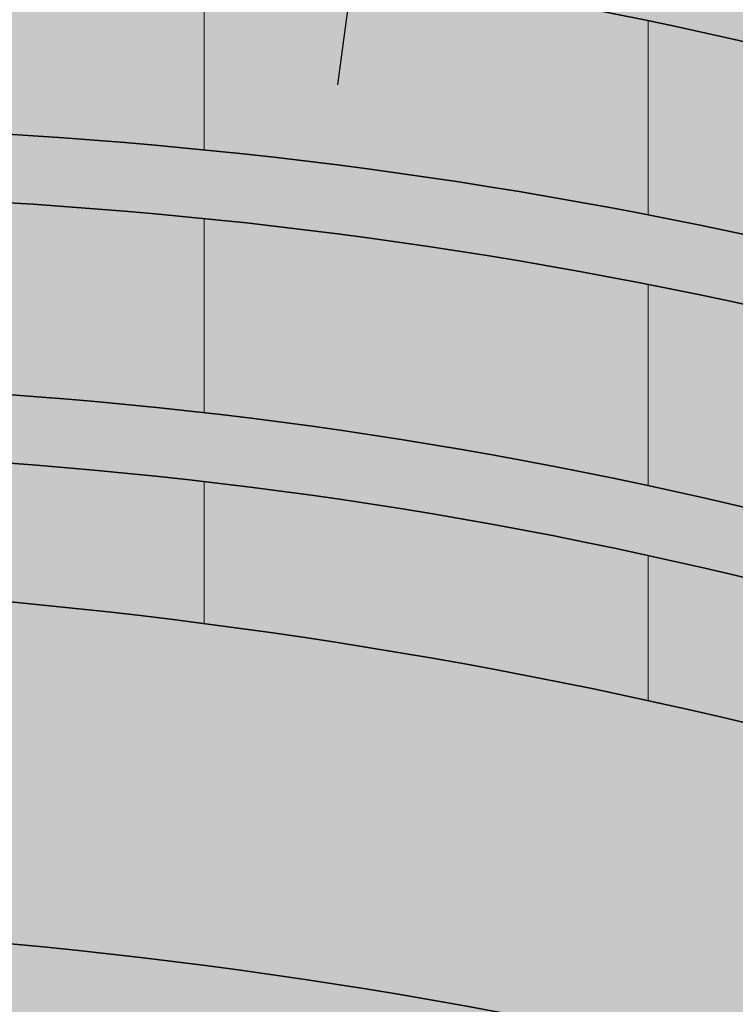
# Model space of a CAD drawing. Units: millimetres. Extents: x 130 to 1021, y 147 to 699.
# Tile 25 of 40: x 442 to 463, y 477 to 505. Entities that reach past the tile are written whole.
import ezdxf

# ---------------------------------------------------------------- set-up
doc = ezdxf.new("R2010")
doc.units = ezdxf.units.MM
doc.header["$MEASUREMENT"] = 0
for name, color, linetype, lineweight in [('A-ANNO-DIMS', 2, 'Continuous', 18), ('A-ELEV', 7, 'Continuous', 35), ('A-ELEV-PATT', 9, 'Continuous', 13), ('A-ELEV-RAIL', 6, 'Continuous', 18)]:
    doc.layers.add(name, color=color, linetype=linetype, lineweight=lineweight)
doc.styles.get("Standard").update_dxf_attribs({"font": 'arial.ttf'})
doc.dimstyles.get("Standard").update_dxf_attribs({"dimtxt": 20, "dimasz": 10, "dimexe": 10, "dimexo": 10, "dimgap": 5, "dimtad": 0, "dimtih": 1, "dimtoh": 1, "dimdec": 0, "dimzin": 0, "dimdsep": 46, "dimtxsty": 'Standard', "dimcen": 5, "dimadec": 0, "dimazin": 0, "dimtfac": 1, "dimtdec": 0, "dimtofl": 0, "dimtmove": 0, "dimatfit": 3, "dimfxl": 1, "dimtolj": 1, "dimtzin": 0, "dimarcsym": 0})

# ---------------------------------------------------------------- blocks, each defined once
blk = doc.blocks.new('*D11')
at = {"layer": 'A-ANNO-DIMS', "color": 0, "lineweight": -2, "transparency": 16777216}
for p, q in [((737.374, 648.699), (737.374, 149.739)), ((299.374, 566.947), (299.374, 149.739)), ((309.374, 159.739), (490.857, 159.739)), ((727.374, 159.739), (545.891, 159.739))]:
    blk.add_line(p, q, dxfattribs=at)
at = {"layer": 'A-ANNO-DIMS', "color": 0, "transparency": 16777216}
for points in [[(309.374, 161.406), (309.374, 158.073), (299.374, 159.739)], [(727.374, 161.406), (727.374, 158.073), (737.374, 159.739)]]:
    blk.add_solid(points, dxfattribs=at)
at = {"layer": 'Defpoints', "color": 0, "transparency": 16777216}
for p in [(737.374, 658.699), (299.374, 576.947), (737.374, 159.739)]:
    blk.add_point(p, dxfattribs=at)
at = {"layer": 'A-ANNO-DIMS', "color": 0, "transparency": 16777216, "insert": (518.374, 159.739), "char_height": 20, "attachment_point": 5}
blk.add_mtext('\\A1;438', dxfattribs=at)
blk = doc.blocks.new('*D12')
at = {"layer": 'A-ANNO-DIMS', "color": 0, "lineweight": -2, "transparency": 16777216}
for p, q in [((477.374, 661.947), (265.074, 661.947)), ((275.074, 651.947), (275.074, 438.205)), ((275.074, 194.039), (275.074, 407.782)), ((357.163, 184.039), (265.074, 184.039))]:
    blk.add_line(p, q, dxfattribs=at)
at = {"layer": 'A-ANNO-DIMS', "color": 0, "transparency": 16777216}
for points in [[(273.407, 651.947), (276.74, 651.947), (275.074, 661.947)], [(273.407, 194.039), (276.74, 194.039), (275.074, 184.039)]]:
    blk.add_solid(points, dxfattribs=at)
at = {"layer": 'Defpoints', "color": 0, "transparency": 16777216}
for p in [(275.074, 661.947), (487.374, 661.947), (367.163, 184.039)]:
    blk.add_point(p, dxfattribs=at)
at = {"layer": 'A-ANNO-DIMS', "color": 0, "transparency": 16777216, "insert": (275.074, 422.993), "char_height": 20, "attachment_point": 5}
blk.add_mtext('\\A1;477.9', dxfattribs=at)
blk = doc.blocks.new('*D16')
at = {"layer": 'A-ANNO-DIMS', "color": 0, "lineweight": -2, "transparency": 16777216}
for p, q in [((357.941, 411.947), (357.941, 696.247)), ((363.922, 579.884), (363.922, 696.247)), ((347.941, 686.247), (337.941, 686.247)), ((373.922, 686.247), (383.922, 686.247))]:
    blk.add_line(p, q, dxfattribs=at)
at = {"layer": 'A-ANNO-DIMS', "color": 0, "transparency": 16777216}
for points in [[(347.941, 687.914), (347.941, 684.581), (357.941, 686.247)], [(373.922, 687.914), (373.922, 684.581), (363.922, 686.247)]]:
    blk.add_solid(points, dxfattribs=at)
at = {"layer": 'Defpoints', "color": 0, "transparency": 16777216}
for p in [(363.922, 686.247), (363.922, 569.884), (357.941, 401.947)]:
    blk.add_point(p, dxfattribs=at)
at = {"layer": 'A-ANNO-DIMS', "color": 0, "transparency": 16777216, "insert": (420.737, 686.247), "char_height": 20, "attachment_point": 5}
blk.add_mtext('\\A1;5.981', dxfattribs=at)
blk = doc.blocks.new('*D17')
at = {"layer": 'A-ANNO-DIMS', "color": 0, "lineweight": -2, "transparency": 16777216}
for p, q in [((363.922, 579.884), (363.922, 696.247)), ((375.85, 490.216), (375.85, 696.247)), ((353.922, 686.247), (343.922, 686.247)), ((385.85, 686.247), (395.85, 686.247))]:
    blk.add_line(p, q, dxfattribs=at)
at = {"layer": 'A-ANNO-DIMS', "color": 0, "transparency": 16777216}
for points in [[(353.922, 687.914), (353.922, 684.581), (363.922, 686.247)], [(385.85, 687.914), (385.85, 684.581), (375.85, 686.247)]]:
    blk.add_solid(points, dxfattribs=at)
at = {"layer": 'Defpoints', "color": 0, "transparency": 16777216}
for p in [(375.85, 686.247), (363.922, 569.884), (375.85, 480.216)]:
    blk.add_point(p, dxfattribs=at)
at = {"layer": 'A-ANNO-DIMS', "color": 0, "transparency": 16777216, "insert": (441.444, 686.247), "char_height": 20, "attachment_point": 5}
blk.add_mtext('\\A1;11.928', dxfattribs=at)
blk = doc.blocks.new('*D18')
at = {"layer": 'A-ANNO-DIMS', "color": 0, "lineweight": -2, "transparency": 16777216}
for p, q in [((375.85, 490.216), (375.85, 696.247)), ((382.374, 388.947), (382.374, 696.247)), ((365.85, 686.247), (355.85, 686.247)), ((392.374, 686.247), (402.374, 686.247))]:
    blk.add_line(p, q, dxfattribs=at)
at = {"layer": 'A-ANNO-DIMS', "color": 0, "transparency": 16777216}
for points in [[(365.85, 687.914), (365.85, 684.581), (375.85, 686.247)], [(392.374, 687.914), (392.374, 684.581), (382.374, 686.247)]]:
    blk.add_solid(points, dxfattribs=at)
at = {"layer": 'Defpoints', "color": 0, "transparency": 16777216}
for p in [(382.374, 686.247), (375.85, 480.216), (382.374, 378.947)]:
    blk.add_point(p, dxfattribs=at)
at = {"layer": 'A-ANNO-DIMS', "color": 0, "transparency": 16777216, "insert": (441.132, 686.247), "char_height": 20, "attachment_point": 5}
blk.add_mtext('\\A1;6.524', dxfattribs=at)
blk = doc.blocks.new('*D19')
at = {"layer": 'A-ANNO-DIMS', "color": 0, "lineweight": -2, "transparency": 16777216}
for p, q in [((382.374, 388.947), (382.374, 696.247)), ((414.652, 510.881), (414.652, 696.247)), ((392.374, 686.247), (404.652, 686.247)), ((414.652, 686.247), (424.652, 686.247))]:
    blk.add_line(p, q, dxfattribs=at)
at = {"layer": 'A-ANNO-DIMS', "color": 0, "transparency": 16777216}
for points in [[(392.374, 687.914), (392.374, 684.581), (382.374, 686.247)], [(404.652, 687.914), (404.652, 684.581), (414.652, 686.247)]]:
    blk.add_solid(points, dxfattribs=at)
at = {"layer": 'Defpoints', "color": 0, "transparency": 16777216}
for p in [(414.652, 686.247), (414.652, 500.881), (382.374, 378.947)]:
    blk.add_point(p, dxfattribs=at)
at = {"layer": 'A-ANNO-DIMS', "color": 0, "transparency": 16777216, "insert": (463.411, 686.247), "char_height": 20, "attachment_point": 5}
blk.add_mtext('\\A1;32.28', dxfattribs=at)
blk = doc.blocks.new('*D20')
at = {"layer": 'A-ANNO-DIMS', "color": 0, "lineweight": -2, "transparency": 16777216}
for p, q in [((414.652, 510.881), (414.652, 696.247)), ((432.374, 388.947), (432.374, 696.247)), ((404.652, 686.247), (394.652, 686.247)), ((442.374, 686.247), (452.374, 686.247))]:
    blk.add_line(p, q, dxfattribs=at)
at = {"layer": 'A-ANNO-DIMS', "color": 0, "transparency": 16777216}
for points in [[(404.652, 687.914), (404.652, 684.581), (414.652, 686.247)], [(442.374, 687.914), (442.374, 684.581), (432.374, 686.247)]]:
    blk.add_solid(points, dxfattribs=at)
at = {"layer": 'Defpoints', "color": 0, "transparency": 16777216}
for p in [(432.374, 686.247), (414.652, 500.881), (432.374, 378.947)]:
    blk.add_point(p, dxfattribs=at)
at = {"layer": 'A-ANNO-DIMS', "color": 0, "transparency": 16777216, "insert": (490.075, 686.247), "char_height": 20, "attachment_point": 5}
blk.add_mtext('\\A1;17.72', dxfattribs=at)
blk = doc.blocks.new('*D21')
at = {"layer": 'A-ANNO-DIMS', "color": 0, "lineweight": -2, "transparency": 16777216}
for p, q in [((432.374, 388.947), (432.374, 696.247)), ((447.374, 656.947), (447.374, 696.247)), ((422.374, 686.247), (412.374, 686.247)), ((457.374, 686.247), (467.374, 686.247))]:
    blk.add_line(p, q, dxfattribs=at)
at = {"layer": 'A-ANNO-DIMS', "color": 0, "transparency": 16777216}
for points in [[(422.374, 687.914), (422.374, 684.581), (432.374, 686.247)], [(457.374, 687.914), (457.374, 684.581), (447.374, 686.247)]]:
    blk.add_solid(points, dxfattribs=at)
at = {"layer": 'Defpoints', "color": 0, "transparency": 16777216}
for p in [(447.374, 686.247), (447.374, 646.947), (432.374, 378.947)]:
    blk.add_point(p, dxfattribs=at)
at = {"layer": 'A-ANNO-DIMS', "color": 0, "transparency": 16777216, "insert": (485.832, 686.247), "char_height": 20, "attachment_point": 5}
blk.add_mtext('\\A1;15', dxfattribs=at)
blk = doc.blocks.new('*D22')
at = {"layer": 'A-ANNO-DIMS', "color": 0, "lineweight": -2, "transparency": 16777216}
for p, q in [((447.374, 656.947), (447.374, 696.247)), ((466.767, 403.947), (466.767, 696.247)), ((437.374, 686.247), (427.374, 686.247)), ((476.767, 686.247), (486.767, 686.247))]:
    blk.add_line(p, q, dxfattribs=at)
at = {"layer": 'A-ANNO-DIMS', "color": 0, "transparency": 16777216}
for points in [[(437.374, 687.914), (437.374, 684.581), (447.374, 686.247)], [(476.767, 687.914), (476.767, 684.581), (466.767, 686.247)]]:
    blk.add_solid(points, dxfattribs=at)
at = {"layer": 'Defpoints', "color": 0, "transparency": 16777216}
for p in [(466.767, 686.247), (447.374, 646.947), (466.767, 393.947)]:
    blk.add_point(p, dxfattribs=at)
at = {"layer": 'A-ANNO-DIMS', "color": 0, "transparency": 16777216, "insert": (532.34, 686.247), "char_height": 20, "attachment_point": 5}
blk.add_mtext('\\A1;19.393', dxfattribs=at)
blk = doc.blocks.new('*D23')
at = {"layer": 'A-ANNO-DIMS', "color": 0, "lineweight": -2, "transparency": 16777216}
for p, q in [((466.767, 403.947), (466.767, 696.247)), ((475.988, 209.039), (475.988, 696.247)), ((456.767, 686.247), (446.767, 686.247)), ((485.988, 686.247), (495.988, 686.247))]:
    blk.add_line(p, q, dxfattribs=at)
at = {"layer": 'A-ANNO-DIMS', "color": 0, "transparency": 16777216}
for points in [[(456.767, 687.914), (456.767, 684.581), (466.767, 686.247)], [(485.988, 687.914), (485.988, 684.581), (475.988, 686.247)]]:
    blk.add_solid(points, dxfattribs=at)
at = {"layer": 'Defpoints', "color": 0, "transparency": 16777216}
for p in [(475.988, 686.247), (466.767, 393.947), (475.988, 199.039)]:
    blk.add_point(p, dxfattribs=at)
at = {"layer": 'A-ANNO-DIMS', "color": 0, "transparency": 16777216, "insert": (534.631, 686.247), "char_height": 20, "attachment_point": 5}
blk.add_mtext('\\A1;9.222', dxfattribs=at)
blk = doc.blocks.new('*D24')
at = {"layer": 'A-ANNO-DIMS', "color": 0, "lineweight": -2, "transparency": 16777216}
for p, q in [((475.988, 209.039), (475.988, 696.247)), ((487.374, 671.947), (487.374, 696.247)), ((465.988, 686.247), (455.988, 686.247)), ((497.374, 686.247), (507.374, 686.247))]:
    blk.add_line(p, q, dxfattribs=at)
at = {"layer": 'A-ANNO-DIMS', "color": 0, "transparency": 16777216}
for points in [[(465.988, 687.914), (465.988, 684.581), (475.988, 686.247)], [(497.374, 687.914), (497.374, 684.581), (487.374, 686.247)]]:
    blk.add_solid(points, dxfattribs=at)
at = {"layer": 'Defpoints', "color": 0, "transparency": 16777216}
for p in [(487.374, 686.247), (487.374, 661.947), (475.988, 199.039)]:
    blk.add_point(p, dxfattribs=at)
at = {"layer": 'A-ANNO-DIMS', "color": 0, "transparency": 16777216, "insert": (553.022, 686.247), "char_height": 20, "attachment_point": 5}
blk.add_mtext('\\A1;11.385', dxfattribs=at)
blk = doc.blocks.new('*D65')
at = {"layer": 'A-ANNO-DIMS', "color": 0, "lineweight": -2, "transparency": 16777216}
for p, q in [((495.463, 509.127), (472.508, 423.108)), ((505.463, 509.127), (495.463, 509.127)), ((427.374, 248.979), (427.374, 258.979)), ((422.374, 253.979), (432.374, 253.979))]:
    blk.add_line(p, q, dxfattribs=at)
at = {"layer": 'A-ANNO-DIMS', "color": 0, "transparency": 16777216}
blk.add_solid([(470.898, 423.538), (474.118, 422.679), (469.93, 413.447)], dxfattribs=at)
at = {"layer": 'Defpoints', "color": 0, "transparency": 16777216}
for p in [(469.93, 413.447), (427.374, 253.979)]:
    blk.add_point(p, dxfattribs=at)
at = {"layer": 'A-ANNO-DIMS', "color": 0, "transparency": 16777216, "insert": (561.623, 509.127), "char_height": 20, "attachment_point": 5}
blk.add_mtext('\\A1;R165.05', dxfattribs=at)
blk = doc.blocks.new('*D67')
at = {"layer": 'A-ANNO-DIMS', "color": 0, "lineweight": -2, "transparency": 16777216}
for p, q in [((479.756, 492.431), (462.144, 412.223)), ((489.756, 492.431), (479.756, 492.431)), ((427.07, 247.496), (427.07, 257.496)), ((422.07, 252.496), (432.07, 252.496))]:
    blk.add_line(p, q, dxfattribs=at)
at = {"layer": 'A-ANNO-DIMS', "color": 0, "transparency": 16777216}
blk.add_solid([(460.516, 412.58), (463.772, 411.865), (459.999, 402.455)], dxfattribs=at)
at = {"layer": 'Defpoints', "color": 0, "transparency": 16777216}
for p in [(459.999, 402.455), (427.07, 252.496)]:
    blk.add_point(p, dxfattribs=at)
at = {"layer": 'A-ANNO-DIMS', "color": 0, "transparency": 16777216, "insert": (545.841, 492.431), "char_height": 20, "attachment_point": 5}
blk.add_mtext('\\A1;R153.53', dxfattribs=at)
blk = doc.blocks.new('*D69')
at = {"layer": 'A-ANNO-DIMS', "color": 0, "lineweight": -2, "transparency": 16777216}
for p, q in [((507.746, 572.261), (483.091, 501.813)), ((517.746, 572.261), (507.746, 572.261)), ((433.191, 354.23), (433.191, 364.23)), ((428.191, 359.23), (438.191, 359.23))]:
    blk.add_line(p, q, dxfattribs=at)
at = {"layer": 'A-ANNO-DIMS', "color": 0, "transparency": 16777216}
blk.add_solid([(481.518, 502.363), (484.664, 501.262), (479.788, 492.374)], dxfattribs=at)
at = {"layer": 'Defpoints', "color": 0, "transparency": 16777216}
for p in [(479.788, 492.374), (433.191, 359.23)]:
    blk.add_point(p, dxfattribs=at)
at = {"layer": 'A-ANNO-DIMS', "color": 0, "transparency": 16777216, "insert": (573.824, 572.261), "char_height": 20, "attachment_point": 5}
blk.add_mtext('\\A1;R141.06', dxfattribs=at)
blk = doc.blocks.new('*D71')
at = {"layer": 'A-ANNO-DIMS', "color": 0, "lineweight": -2, "transparency": 16777216}
for p, q in [((492.108, 581.609), (472.542, 512.666)), ((502.108, 581.609), (492.108, 581.609)), ((432.65, 367.109), (432.65, 377.109)), ((427.65, 372.109), (437.65, 372.109))]:
    blk.add_line(p, q, dxfattribs=at)
at = {"layer": 'A-ANNO-DIMS', "color": 0, "transparency": 16777216}
blk.add_solid([(470.938, 513.121), (474.145, 512.211), (469.812, 503.046)], dxfattribs=at)
at = {"layer": 'Defpoints', "color": 0, "transparency": 16777216}
for p in [(469.812, 503.046), (432.65, 372.109)]:
    blk.add_point(p, dxfattribs=at)
at = {"layer": 'A-ANNO-DIMS', "color": 0, "transparency": 16777216, "insert": (548.493, 581.609), "char_height": 20, "attachment_point": 5}
blk.add_mtext('\\A1;R136.1', dxfattribs=at)
blk = doc.blocks.new('*D72')
at = {"layer": 'A-ANNO-DIMS', "color": 0, "lineweight": -2, "transparency": 16777216}
for p, q in [((460.658, 573.64), (451.279, 503.49)), ((470.658, 573.64), (460.658, 573.64)), ((432.115, 355.142), (432.115, 365.142)), ((427.115, 360.142), (437.115, 360.142))]:
    blk.add_line(p, q, dxfattribs=at)
at = {"layer": 'A-ANNO-DIMS', "color": 0, "transparency": 16777216}
blk.add_solid([(449.628, 503.711), (452.931, 503.27), (449.954, 493.579)], dxfattribs=at)
at = {"layer": 'Defpoints', "color": 0, "transparency": 16777216}
for p in [(449.954, 493.579), (432.115, 360.142)]:
    blk.add_point(p, dxfattribs=at)
at = {"layer": 'A-ANNO-DIMS', "color": 0, "transparency": 16777216, "insert": (526.64, 573.64), "char_height": 20, "attachment_point": 5}
blk.add_mtext('\\A1;R134.62', dxfattribs=at)

msp = doc.modelspace()

# ---------------------------------------------------------------- hatches: boundary and pattern name
at = {"layer": 'A-ELEV-PATT'}
h = msp.add_hatch(color=256, dxfattribs=at)
h.dxf.hatch_style = 1
h.paths.add_polyline_path([(737.3738, 658.6988, 0.0135961), (632.4019, 661.9473), (607.3738, 661.9473), (487.3738, 661.9473), (487.3738, 649.9473), (607.3738, 649.9473), (632.3794, 649.9473, -0.0136841), (737.3738, 646.6784)])
h.paths.add_polyline_path([(732.3738, 643.9599, 0.0130529), (632.3738, 646.9473), (607.3738, 646.9473), (487.3738, 646.9473), (487.3738, 596.9473), (632.3738, 596.9473, -0.0130529), (732.3738, 593.9599)])
h.paths.add_polyline_path([(737.3738, 593.6732, 0.0137063), (632.3738, 596.9473), (487.3738, 596.9473), (487.3738, 586.9473), (632.355, 586.9473, -0.0137808), (737.3738, 583.6559)])
h.paths.add_polyline_path([(447.3738, 646.9473), (307.3738, 646.9473), (302.3738, 646.9473), (302.3738, 634.9473), (447.3738, 634.9473)])
h.paths.add_polyline_path([(447.3738, 631.9473), (307.3738, 631.9473), (307.3738, 586.9473), (447.3738, 586.9473)])
h.paths.add_polyline_path([(447.3738, 586.9473), (307.3738, 586.9473), (302.3738, 586.9473), (302.3738, 576.9473), (447.3738, 576.9473)])
h.paths.add_polyline_path([(447.3738, 573.9473), (367.3738, 573.9473), (367.3738, 539.9473), (447.3738, 539.9473)])
h.paths.add_polyline_path([(447.3738, 537.9473), (367.3738, 537.9473), (367.3738, 507.9473), (400.392, 507.4253, -0.001728), (401.3281, 507.6451, -0.5220025), (425.6117, 511.0391, -0.0391849), (447.3738, 510.4359), (447.3738, 510.7883)])
h.paths.add_polyline_path([(394.7238, 505.9473), (367.3738, 505.9473), (367.3738, 476.9473, -0.0146512), (375.8501, 480.2159), (376.1506, 499.2266, -0.0355419)])
h.paths.add_polyline_path([(632.3738, 583.9473), (552.3738, 583.9473), (552.3738, 550.9473), (632.3738, 550.9473)])
h.paths.add_polyline_path([(632.3738, 548.9473), (552.3738, 548.9473), (552.3738, 515.9473), (632.3738, 515.9473)])
h.paths.add_polyline_path([(632.3738, 513.9473), (552.3738, 513.9473), (552.3738, 476.9473), (632.3738, 476.9473)])
h.paths.add_polyline_path([(737.3738, 473.6903, 0.0136326), (632.3926, 476.9473), (552.3738, 476.9473), (487.3738, 476.9473), (487.3738, 466.9473), (632.3738, 466.9473, -0.0137063), (737.3738, 463.6732)])
h.paths.add_polyline_path([(732.3738, 460.9552, 0.0130741), (632.3681, 463.9473), (487.3738, 463.9473), (487.3738, 407.735, -0.0032286), (489.3544, 406.9473), (632.3926, 406.9473, -0.0129826), (732.3738, 403.9755)])
h.paths.add_polyline_path([(487.3738, 463.9473, 0.20133), (367.3738, 463.9473), (367.3738, 407.735, -0.1882031), (487.3738, 407.735)])
h.paths.add_polyline_path([(367.3738, 476.9473), (367.3738, 466.9473, -0.2013309), (487.3738, 466.9473), (487.3738, 476.9473, 0.20133)])
h.paths.add_polyline_path([(367.3738, 463.9473), (307.3738, 463.9473), (307.3738, 401.9473), (357.9413, 401.9473), (367.3738, 407.735)])
h.paths.add_polyline_path([(367.3738, 476.9473), (302.3738, 476.9473), (302.3738, 466.9473), (367.3738, 466.9473)])
h.paths.add_polyline_path([(632.8184, 366.9453), (552.3738, 366.9453), (552.3738, 393.9473), (632.8184, 393.9473)])
h.paths.add_polyline_path([(632.8184, 357.2114), (632.8184, 363.9453), (552.3738, 363.9453), (552.3738, 357.2114), (552.3738, 336.9453), (632.8184, 336.9453)])
h.paths.add_polyline_path([(632.8184, 333.9453), (552.3738, 333.9453), (552.3738, 306.9453), (632.8184, 306.9453)])
h.paths.add_polyline_path([(632.8184, 303.9453), (552.3738, 303.9453), (552.3738, 273.9473), (632.355, 273.9473, 0.0000608), (632.8184, 273.9491)])
h.paths.add_polyline_path([(737.3738, 403.6903, 0.0136326), (632.3926, 406.9473), (489.3544, 406.9473, 0.1915481), (367.3738, 407.735), (367.3738, 396.9473, -0.2013309), (487.3738, 396.9473), (632.3738, 396.9473, -0.0137063), (737.3738, 393.6732)])
h.paths.add_polyline_path([(357.9413, 401.9473), (307.3738, 401.9473), (307.3738, 391.9473), (357.9413, 391.9473)])
h.paths.add_polyline_path([(357.9413, 357.2114), (357.9413, 388.9473), (307.3738, 388.9473), (307.3738, 357.2114), (307.3738, 273.9473), (357.9413, 273.9473)])
h.paths.add_polyline_path([(732.3738, 263.93, -0.0130317), (632.3794, 260.9473), (466.7667, 260.9473), (466.7667, 240.9473), (469.8406, 236.978), (469.8406, 221.978), (472.9145, 218.0087), (472.9145, 213.9473), (607.3738, 213.9473), (732.3738, 213.9473)])
h.paths.add_polyline_path([(732.3738, 290.889), (722.479, 290.889), (722.479, 301.889), (732.3738, 301.889), (732.3738, 305.889), (722.479, 305.889), (722.479, 316.889), (732.3738, 316.889), (732.3738, 320.889), (722.479, 320.889), (722.479, 331.889), (732.3738, 331.889), (732.3738, 335.889), (722.479, 335.889), (722.479, 346.889), (732.3738, 346.889), (732.3738, 350.889), (722.479, 350.889), (722.479, 361.889), (732.3738, 361.889), (732.3738, 365.889), (722.479, 365.889), (722.479, 376.889), (732.3738, 376.889), (732.3738, 380.889), (722.479, 380.889), (722.479, 391.4848, 0.0005233), (718.479, 391.6843), (718.479, 380.889), (707.479, 380.889), (707.479, 392.1896, 0.0005231), (703.479, 392.3576), (703.479, 380.889), (692.479, 380.889), (692.479, 392.7765, 0.0005229), (688.479, 392.9131), (688.479, 380.889), (677.479, 380.889), (677.479, 393.2456, 0.0005228), (673.479, 393.3508), (673.479, 380.889), (662.479, 380.889), (662.479, 393.597, 0.0005227), (658.479, 393.6709), (658.479, 380.889), (647.479, 380.889), (647.479, 393.8308, 0.0005226), (643.479, 393.8732), (643.479, 380.889), (632.8184, 380.889), (632.8184, 376.889), (643.479, 376.889), (643.479, 365.889), (632.8184, 365.889), (632.8184, 361.889), (643.479, 361.889), (643.479, 350.889), (632.8184, 350.889), (632.8184, 346.889), (643.479, 346.889), (643.479, 335.889), (632.8184, 335.889), (632.8184, 331.889), (643.479, 331.889), (643.479, 320.889), (632.8184, 320.889), (632.8184, 316.889), (643.479, 316.889), (643.479, 305.889), (632.8184, 305.889), (632.8184, 301.889), (643.479, 301.889), (643.479, 290.889), (632.8184, 290.889), (632.8184, 286.889), (643.479, 286.889), (643.479, 274.0217, 0.0005246), (647.479, 274.0643), (647.479, 286.889), (658.479, 286.889), (658.479, 274.2248, 0.0005246), (662.479, 274.2989), (662.479, 286.889), (673.479, 286.889), (673.479, 274.546, 0.0005247), (677.479, 274.6516), (677.479, 286.889), (688.479, 286.889), (688.479, 274.9853, 0.0005248), (692.479, 275.1224), (692.479, 286.889), (703.479, 286.889), (703.479, 275.5429, 0.000525), (707.479, 275.7115), (707.479, 286.889), (718.479, 286.889), (718.479, 276.2187, 0.0005252), (722.479, 276.4189), (722.479, 286.889), (732.3738, 286.889)])
h.paths.add_polyline_path([(718.479, 290.889), (707.479, 290.889), (707.479, 301.889), (718.479, 301.889)], flags=16)
h.paths.add_polyline_path([(703.479, 290.889), (692.479, 290.889), (692.479, 301.889), (703.479, 301.889)], flags=16)
h.paths.add_polyline_path([(718.479, 305.889), (707.479, 305.889), (707.479, 316.889), (718.479, 316.889)], flags=16)
h.paths.add_polyline_path([(703.479, 305.889), (692.479, 305.889), (692.479, 316.889), (703.479, 316.889)], flags=16)
h.paths.add_polyline_path([(688.479, 290.889), (677.479, 290.889), (677.479, 301.889), (688.479, 301.889)], flags=16)
h.paths.add_polyline_path([(718.479, 320.889), (707.479, 320.889), (707.479, 331.889), (718.479, 331.889)], flags=16)
h.paths.add_polyline_path([(688.479, 305.889), (677.479, 305.889), (677.479, 316.889), (688.479, 316.889)], flags=16)
h.paths.add_polyline_path([(703.479, 320.889), (692.479, 320.889), (692.479, 331.889), (703.479, 331.889)], flags=16)
h.paths.add_polyline_path([(688.479, 320.889), (677.479, 320.889), (677.479, 331.889), (688.479, 331.889)], flags=16)
h.paths.add_polyline_path([(673.479, 290.889), (662.479, 290.889), (662.479, 301.889), (673.479, 301.889)], flags=16)
h.paths.add_polyline_path([(718.479, 335.889), (707.479, 335.889), (707.479, 346.889), (718.479, 346.889)], flags=16)
h.paths.add_polyline_path([(673.479, 305.889), (662.479, 305.889), (662.479, 316.889), (673.479, 316.889)], flags=16)
h.paths.add_polyline_path([(703.479, 335.889), (692.479, 335.889), (692.479, 346.889), (703.479, 346.889)], flags=16)
h.paths.add_polyline_path([(673.479, 320.889), (662.479, 320.889), (662.479, 331.889), (673.479, 331.889)], flags=16)
h.paths.add_polyline_path([(688.479, 335.889), (677.479, 335.889), (677.479, 346.889), (688.479, 346.889)], flags=16)
h.paths.add_polyline_path([(658.479, 290.889), (647.479, 290.889), (647.479, 301.889), (658.479, 301.889)], flags=16)
h.paths.add_polyline_path([(718.479, 350.889), (707.479, 350.889), (707.479, 361.889), (718.479, 361.889)], flags=16)
h.paths.add_polyline_path([(658.479, 305.889), (647.479, 305.889), (647.479, 316.889), (658.479, 316.889)], flags=16)
h.paths.add_polyline_path([(703.479, 350.889), (692.479, 350.889), (692.479, 361.889), (703.479, 361.889)], flags=16)
h.paths.add_polyline_path([(673.479, 335.889), (662.479, 335.889), (662.479, 346.889), (673.479, 346.889)], flags=16)
h.paths.add_polyline_path([(658.479, 320.889), (647.479, 320.889), (647.479, 331.889), (658.479, 331.889)], flags=16)
h.paths.add_polyline_path([(688.479, 350.889), (677.479, 350.889), (677.479, 361.889), (688.479, 361.889)], flags=16)
h.paths.add_polyline_path([(718.479, 365.889), (707.479, 365.889), (707.479, 376.889), (718.479, 376.889)], flags=16)
h.paths.add_polyline_path([(658.479, 335.889), (647.479, 335.889), (647.479, 346.889), (658.479, 346.889)], flags=16)
h.paths.add_polyline_path([(673.479, 350.889), (662.479, 350.889), (662.479, 361.889), (673.479, 361.889)], flags=16)
h.paths.add_polyline_path([(703.479, 365.889), (692.479, 365.889), (692.479, 376.889), (703.479, 376.889)], flags=16)
h.paths.add_polyline_path([(688.479, 365.889), (677.479, 365.889), (677.479, 376.889), (688.479, 376.889)], flags=16)
h.paths.add_polyline_path([(658.479, 350.889), (647.479, 350.889), (647.479, 361.889), (658.479, 361.889)], flags=16)
h.paths.add_polyline_path([(673.479, 365.889), (662.479, 365.889), (662.479, 376.889), (673.479, 376.889)], flags=16)
h.paths.add_polyline_path([(658.479, 365.889), (647.479, 365.889), (647.479, 376.889), (658.479, 376.889)], flags=16)
h.paths.add_polyline_path([(732.3738, 503.9786), (722.3392, 503.9786), (722.3392, 514.9786), (732.3738, 514.9786), (732.3738, 518.9786), (722.3392, 518.9786), (722.3392, 529.9786), (732.3738, 529.9786), (732.3738, 533.9786), (722.3392, 533.9786), (722.3392, 544.9786), (732.3738, 544.9786), (732.3738, 546.9473), (732.3738, 548.9786), (722.3392, 548.9786), (722.3392, 559.9786), (732.3738, 559.9786), (732.3738, 563.9786), (722.3392, 563.9786), (722.3392, 574.9786), (732.3738, 574.9786), (732.3738, 578.9786), (722.3392, 578.9786), (722.3392, 581.4789, 0.000526), (718.3392, 581.6791), (718.3392, 578.9786), (707.3392, 578.9786), (707.3392, 582.1863, 0.0005258), (703.3392, 582.355), (703.3392, 578.9786), (692.3392, 578.9786), (692.3392, 582.7752, 0.0005257), (688.3392, 582.9123), (688.3392, 578.9786), (677.3392, 578.9786), (677.3392, 583.2457, 0.0005255), (673.3392, 583.3512), (673.3392, 578.9786), (662.3392, 578.9786), (662.3392, 583.5978, 0.0005254), (658.3392, 583.6718), (658.3392, 578.9786), (647.3392, 578.9786), (647.3392, 583.8317, 0.0005254), (643.3392, 583.8741), (643.3392, 578.9786), (632.3738, 578.9786), (632.3738, 574.9786), (643.3392, 574.9786), (643.3392, 563.9786), (632.3738, 563.9786), (632.3738, 559.9786), (643.3392, 559.9786), (643.3392, 548.9786), (632.3738, 548.9786), (632.3738, 544.9786), (643.3392, 544.9786), (643.3392, 533.9786), (632.3738, 533.9786), (632.3738, 529.9786), (643.3392, 529.9786), (643.3392, 518.9786), (632.3738, 518.9786), (632.3738, 515.9473), (632.3738, 514.9786), (643.3392, 514.9786), (643.3392, 503.9786), (632.3738, 503.9786), (632.3738, 499.9786), (643.3392, 499.9786), (643.3392, 488.9786), (632.3738, 488.9786), (632.3738, 484.9786), (643.3392, 484.9786), (643.3392, 476.8751, -0.0005191), (647.3392, 476.8332), (647.3392, 484.9786), (658.3392, 484.9786), (658.3392, 476.6752, -0.0005192), (662.3392, 476.6022), (662.3392, 484.9786), (673.3392, 484.9786), (673.3392, 476.3585, -0.0005193), (677.3392, 476.2543), (677.3392, 484.9786), (688.3392, 484.9786), (688.3392, 475.9248, -0.0005194), (692.3392, 475.7894), (692.3392, 484.9786), (703.3392, 484.9786), (703.3392, 475.3741, -0.0005195), (707.3392, 475.2075), (707.3392, 484.9786), (718.3392, 484.9786), (718.3392, 474.7064, -0.0005197), (722.3392, 474.5086), (722.3392, 484.9786), (732.3738, 484.9786), (732.3738, 488.9786), (722.3392, 488.9786), (722.3392, 499.9786), (732.3738, 499.9786)])
h.paths.add_polyline_path([(718.3392, 503.9786), (707.3392, 503.9786), (707.3392, 514.9786), (718.3392, 514.9786)], flags=16)
h.paths.add_polyline_path([(718.3392, 499.9786), (718.3392, 488.9786), (707.3392, 488.9786), (707.3392, 499.9786)], flags=16)
h.paths.add_polyline_path([(718.3392, 518.9786), (707.3392, 518.9786), (707.3392, 529.9786), (718.3392, 529.9786)], flags=16)
h.paths.add_polyline_path([(703.3392, 503.9786), (692.3392, 503.9786), (692.3392, 514.9786), (703.3392, 514.9786)], flags=16)
h.paths.add_polyline_path([(703.3392, 499.9786), (703.3392, 488.9786), (692.3392, 488.9786), (692.3392, 499.9786)], flags=16)
h.paths.add_polyline_path([(703.3392, 518.9786), (692.3392, 518.9786), (692.3392, 529.9786), (703.3392, 529.9786)], flags=16)
h.paths.add_polyline_path([(718.3392, 533.9786), (707.3392, 533.9786), (707.3392, 544.9786), (718.3392, 544.9786)], flags=16)
h.paths.add_polyline_path([(688.3392, 503.9786), (677.3392, 503.9786), (677.3392, 514.9786), (688.3392, 514.9786)], flags=16)
h.paths.add_polyline_path([(688.3392, 499.9786), (688.3392, 488.9786), (677.3392, 488.9786), (677.3392, 499.9786)], flags=16)
h.paths.add_polyline_path([(703.3392, 533.9786), (692.3392, 533.9786), (692.3392, 544.9786), (703.3392, 544.9786)], flags=16)
h.paths.add_polyline_path([(688.3392, 518.9786), (677.3392, 518.9786), (677.3392, 529.9786), (688.3392, 529.9786)], flags=16)
h.paths.add_polyline_path([(688.3392, 533.9786), (677.3392, 533.9786), (677.3392, 544.9786), (688.3392, 544.9786)], flags=16)
h.paths.add_polyline_path([(718.3392, 548.9786), (707.3392, 548.9786), (707.3392, 559.9786), (718.3392, 559.9786)], flags=16)
h.paths.add_polyline_path([(673.3392, 503.9786), (662.3392, 503.9786), (662.3392, 514.9786), (673.3392, 514.9786)], flags=16)
h.paths.add_polyline_path([(673.3392, 499.9786), (673.3392, 488.9786), (662.3392, 488.9786), (662.3392, 499.9786)], flags=16)
h.paths.add_polyline_path([(703.3392, 548.9786), (692.3392, 548.9786), (692.3392, 559.9786), (703.3392, 559.9786)], flags=16)
h.paths.add_polyline_path([(673.3392, 518.9786), (662.3392, 518.9786), (662.3392, 529.9786), (673.3392, 529.9786)], flags=16)
h.paths.add_polyline_path([(688.3392, 548.9786), (677.3392, 548.9786), (677.3392, 559.9786), (688.3392, 559.9786)], flags=16)
h.paths.add_polyline_path([(673.3392, 533.9786), (662.3392, 533.9786), (662.3392, 544.9786), (673.3392, 544.9786)], flags=16)
h.paths.add_polyline_path([(718.3392, 563.9786), (707.3392, 563.9786), (707.3392, 574.9786), (718.3392, 574.9786)], flags=16)
h.paths.add_polyline_path([(658.3392, 503.9786), (647.3392, 503.9786), (647.3392, 514.9786), (658.3392, 514.9786)], flags=16)
h.paths.add_polyline_path([(658.3392, 499.9786), (658.3392, 488.9786), (647.3392, 488.9786), (647.3392, 499.9786)], flags=16)
h.paths.add_polyline_path([(703.3392, 563.9786), (692.3392, 563.9786), (692.3392, 574.9786), (703.3392, 574.9786)], flags=16)
h.paths.add_polyline_path([(658.3392, 518.9786), (647.3392, 518.9786), (647.3392, 529.9786), (658.3392, 529.9786)], flags=16)
h.paths.add_polyline_path([(673.3392, 548.9786), (662.3392, 548.9786), (662.3392, 559.9786), (673.3392, 559.9786)], flags=16)
h.paths.add_polyline_path([(688.3392, 563.9786), (677.3392, 563.9786), (677.3392, 574.9786), (688.3392, 574.9786)], flags=16)
h.paths.add_polyline_path([(658.3392, 533.9786), (647.3392, 533.9786), (647.3392, 544.9786), (658.3392, 544.9786)], flags=16)
h.paths.add_polyline_path([(673.3392, 563.9786), (662.3392, 563.9786), (662.3392, 574.9786), (673.3392, 574.9786)], flags=16)
h.paths.add_polyline_path([(658.3392, 548.9786), (647.3392, 548.9786), (647.3392, 559.9786), (658.3392, 559.9786)], flags=16)
h.paths.add_polyline_path([(658.3392, 563.9786), (647.3392, 563.9786), (647.3392, 574.9786), (658.3392, 574.9786)], flags=16)
h = msp.add_hatch(color=256, dxfattribs=at)
h.dxf.hatch_style = 1
h.paths.add_polyline_path([(447.3738, 576.9473), (302.3738, 576.9473), (302.3738, 573.9473), (447.3738, 573.9473)])
h.paths.add_polyline_path([(487.3738, 583.9473), (487.3738, 586.9473), (447.3738, 576.9473), (447.3738, 573.9473)])
h.paths.add_polyline_path([(632.355, 586.9473), (487.3738, 586.9473), (487.3738, 583.9473), (632.3738, 583.9473), (632.3738, 583.9472, -0.0138), (737.3738, 580.6507), (737.3738, 583.6559, 0.0137808)])
h.paths.add_polyline_path([(367.3738, 466.9473), (302.3738, 466.9473), (302.3738, 463.9473), (367.3738, 463.9473)])
h.paths.add_polyline_path([(487.3738, 463.9473), (487.3738, 466.9473, 0.2013309), (367.3738, 466.9473), (367.3738, 463.9473, -0.20133)])
h.paths.add_polyline_path([(632.3738, 466.9473), (487.3738, 466.9473), (487.3738, 463.9473), (632.3681, 463.9473, -0.0137285), (737.3738, 460.6681), (737.3738, 463.6732, 0.0137063)])
h.paths.add_polyline_path([(632.3738, 396.9473), (487.3738, 396.9473, 0.2013309), (367.3738, 396.9473), (367.3738, 393.9473, -0.2023717), (486.7667, 393.9473), (632.3681, 393.9473, -0.0137285), (737.3738, 390.6681), (737.3738, 393.6732, 0.0137063)])
h.paths.add_polyline_path([(357.9413, 391.9473), (307.3738, 391.9473), (307.3738, 388.9473), (357.9413, 388.9473)])
h.paths.add_polyline_path([(367.3738, 393.9473), (367.3738, 396.9473), (357.9413, 391.924), (357.9413, 388.9473), (358.058, 388.9473)])
h.paths.add_polyline_path([(737.3738, 264.2162), (737.3738, 267.2214, -0.0137063), (632.3738, 263.9473), (463.7667, 263.9473), (466.7667, 260.9473), (632.3794, 260.9473, 0.0136841)])
h.paths.add_polyline_path([(463.7667, 263.9473), (447.3738, 263.9473), (450.3738, 260.9473), (466.7667, 260.9473)])
h.paths.add_polyline_path([(447.3738, 263.9473), (432.3738, 263.9473), (432.3738, 260.9473), (450.3738, 260.9473)])
h.paths.add_polyline_path([(382.3738, 263.9473), (357.9413, 263.9473), (357.9413, 260.9473), (382.3738, 260.9473)])
h.paths.add_polyline_path([(357.9413, 263.9473), (307.3738, 263.9473), (307.3738, 260.9473), (357.9413, 260.9473)])
h = msp.add_hatch(color=256, dxfattribs=at)
h.paths.add_polyline_path([(375.8501, 480.2159, -0.0051389), (378.8667, 481.244), (378.8725, 481.6093, -0.2220519), (491.1023, 478.9257), (491.1023, 476.9473), (494.1023, 476.9473), (494.1023, 496.908, 0.2225165), (376.1506, 499.2266)])
h.paths.add_polyline_path([(379.1197, 497.2486, -0.2152592), (491.1023, 495.0271), (491.1023, 490.0474, 0.2040153), (379.0311, 491.6449)], flags=16)
h.paths.add_polyline_path([(491.1023, 487.8572), (491.1023, 481.1546, 0.1695534), (402.9637, 491.5717, -0.0927216), (400.3891, 496.4261, -0.1659296)], flags=16)
h = msp.add_hatch(color=256, dxfattribs=at)
h.paths.add_polyline_path([(399.9219, 498.3708, -0.0996756), (400.0983, 504.2673, 0.0406995), (379.1197, 497.2486), (379.0311, 491.6449, -0.0384084)])
h.paths.add_polyline_path([(402.9637, 491.5717, -0.0927216), (400.3891, 496.4261, 0.0399321), (378.9967, 489.4672), (378.9072, 483.8048, -0.0470483)])
h.paths.add_polyline_path([(404.5509, 489.8698, 0.0509798), (378.8725, 481.6093), (378.8667, 481.244, -0.0474823), (407.5193, 487.7506, -0.061248)])
h.paths.add_polyline_path([(447.3738, 491.8851, 0.0382282), (427.1388, 492.6724, -0.0850627), (423.6933, 488.9834, -0.0382916), (447.3738, 487.7318)])
h.paths.add_polyline_path([(447.3738, 499.578, 0.0315856), (429.5819, 500.2467, -0.0960946), (428.2619, 494.7107, -0.0355683), (447.3738, 493.8983)])
h.paths.add_polyline_path([(447.3738, 507.4186, 0.0361693), (427.7205, 508.128, -0.1040877), (429.5329, 502.2461, -0.0312283), (447.3738, 501.588)])
h = msp.add_hatch(color=256, dxfattribs=at)
h.paths.add_polyline_path([(463.3738, 504.7044, 0.0056421), (460.3738, 505.364), (460.3738, 499.6866, -0.0053513), (463.3738, 499.0726)])
h.paths.add_polyline_path([(460.3738, 505.364, 0.0241885), (447.3738, 507.4186), (447.3738, 501.588, -0.0229712), (460.3738, 499.6866)])
h.paths.add_polyline_path([(460.3738, 497.6489, 0.0233044), (447.3738, 499.578), (447.3738, 493.8983, -0.0244785), (460.3738, 491.7665)])
h.paths.add_polyline_path([(460.3738, 489.7202, 0.0248583), (447.3738, 491.8851), (447.3738, 487.7318, -0.0212844), (460.3738, 485.4746)])
h.paths.add_polyline_path([(463.3738, 497.0258, 0.0054304), (460.3738, 497.6489), (460.3738, 491.7665, -0.0057126), (463.3738, 491.0865)])
h.paths.add_polyline_path([(463.3738, 489.0294, 0.0058033), (460.3738, 489.7202), (460.3738, 485.4746, -0.0049617), (463.3738, 484.7899)])
h.paths.add_polyline_path([(472.3738, 502.2917, 0.0057416), (469.3738, 503.1695), (469.3738, 497.6415, -0.0054346), (472.3738, 496.8223)])
h.paths.add_polyline_path([(472.3738, 494.7416, 0.0055175), (469.3738, 495.5733), (469.3738, 489.5072, -0.0058176), (472.3738, 488.6052)])
h.paths.add_polyline_path([(472.3738, 486.5077, 0.0059135), (469.3738, 487.4246), (469.3738, 483.2302, -0.0050397), (472.3738, 482.3533)])

# ---------------------------------------------------------------- linework, layer by layer
at = {"layer": 'A-ELEV'}
for centre, radius, start, end in [((432.6505, 372.1087), 139.1086, 63.78413, 113.963624), ((432.6505, 372.1087), 136.1086, 64.567343, 113.15965), ((433.1906, 359.2304), 143.0624, 66.12141, 112.245303), ((433.1906, 359.2304), 141.0624, 65.761287, 112.593106), ((432.115, 360.1423), 134.6235, 64.013142, 113.246941), ((432.115, 360.1423), 132.6235, 63.591208, 113.669232), ((427.3738, 333.9781), 155.049, 67.23363, 112.76637), ((427.3738, 323.9788), 155.0484, 67.233534, 112.766466)]:
    msp.add_arc(centre, radius, start, end, dxfattribs=at)
at = {"layer": 'A-ELEV-RAIL'}
for p, q in [((447.3738, 507.4186), (447.3738, 501.588)), ((460.3738, 505.364), (460.3738, 499.6866)), ((447.3738, 499.578), (447.3738, 493.8983)), ((460.3738, 497.6489), (460.3738, 491.7665)), ((447.3738, 491.8851), (447.3738, 487.7318)), ((460.3738, 489.7202), (460.3738, 485.4746))]:
    msp.add_line(p, q, dxfattribs=at)

# ---------------------------------------------------------------- dimensions: what is measured, and where the dimension line sits
at = {"layer": 'A-ANNO-DIMS'}
for base, p1, p2, override, picture, middle in [((363.922, 686.2473), (357.9413, 401.9473), (363.922, 569.884), {"dimdec": 3, "dimlfac": 1, "dimrnd": 0, "dimzin": 0, "dimdsep": 46, "dimlunit": 2}, '*D16', (420.7365, 686.2473)), ((375.8501, 686.2473), (363.922, 569.884), (375.8501, 480.2159), {"dimdec": 3, "dimlfac": 1, "dimrnd": 0, "dimzin": 0, "dimdsep": 46, "dimlunit": 2}, '*D17', (441.4435, 686.2473)), ((382.3738, 686.2473), (375.8501, 480.2159), (382.3738, 378.9473), {"dimdec": 3, "dimlfac": 1, "dimrnd": 0, "dimzin": 0, "dimdsep": 46, "dimlunit": 2}, '*D18', (441.1323, 686.2473)), ((414.6525, 686.2473), (382.3738, 378.9473), (414.6525, 500.8811), {"dimdec": 2, "dimlfac": 1, "dimrnd": 0, "dimzin": 0, "dimdsep": 46, "dimlunit": 2}, '*D19', (463.411, 686.2473)), ((432.3738, 686.2473), (414.6525, 500.8811), (432.3738, 378.9473), {"dimdec": 2, "dimlfac": 1, "dimrnd": 0, "dimzin": 0, "dimdsep": 46, "dimlunit": 2}, '*D20', (490.075, 686.2473)), ((447.3738, 686.2473), (432.3738, 378.9473), (447.3738, 646.9473), {"dimdec": 0, "dimlfac": 1, "dimrnd": 0, "dimzin": 0, "dimdsep": 46, "dimlunit": 2}, '*D21', (485.8322, 686.2473)), ((466.7667, 686.2473), (447.3738, 646.9473), (466.7667, 393.9473), {"dimdec": 3, "dimlfac": 1, "dimrnd": 0, "dimzin": 0, "dimdsep": 46, "dimlunit": 2}, '*D22', (532.3397, 686.2473)), ((475.9885, 686.2473), (466.7667, 393.9473), (475.9885, 199.0395), {"dimdec": 3, "dimlfac": 1, "dimrnd": 0, "dimzin": 0, "dimdsep": 46, "dimlunit": 2}, '*D23', (534.631, 686.2473)), ((487.3738, 686.2473), (475.9885, 199.0395), (487.3738, 661.9473), {"dimdec": 3, "dimlfac": 1, "dimrnd": 0, "dimzin": 0, "dimdsep": 46, "dimlunit": 2}, '*D24', (553.0218, 686.2473)), ((737.3738, 159.7395), (299.3738, 576.9473), (737.3738, 658.6988), {"dimdec": 0, "dimlfac": 1, "dimrnd": 0, "dimzin": 0, "dimdsep": 46, "dimlunit": 2}, '*D11', (518.3738, 159.7395))]:
    dim = msp.add_linear_dim(base=base, p1=p1, p2=p2, dimstyle='Standard', override=override, dxfattribs=at)
    dim.commit()
    dim.dimension.update_dxf_attribs({"geometry": picture, "text_midpoint": middle})
dim = msp.add_linear_dim(base=(275.0738, 661.9473), p1=(367.163, 184.0395), p2=(487.3738, 661.9473), angle=90, dimstyle='Standard', override={"dimdec": 1, "dimlfac": 1, "dimrnd": 0, "dimzin": 0, "dimdsep": 46, "dimlunit": 2}, dxfattribs=at)
dim.commit()
dim.dimension.update_dxf_attribs({"geometry": '*D12', "text_midpoint": (275.0738, 422.9934)})
for center, mpoint, override, picture, middle in [((432.6505, 372.1087), (469.8116, 503.0461), {"dimdec": 1, "dimlfac": 1, "dimrnd": 0, "dimzin": 0, "dimdsep": 46, "dimlunit": 2}, '*D71', (548.493, 581.6085)), ((432.115, 360.1423), (449.9544, 493.5786), {"dimdec": 2, "dimlfac": 1, "dimrnd": 0, "dimzin": 0, "dimdsep": 46, "dimlunit": 2}, '*D72', (526.6403, 573.6404)), ((433.1906, 359.2304), (479.788, 492.3743), {"dimdec": 2, "dimlfac": 1, "dimrnd": 0, "dimzin": 0, "dimdsep": 46, "dimlunit": 2}, '*D69', (573.8242, 572.2606)), ((427.3738, 253.9788), (469.9297, 413.4465), {"dimdec": 2, "dimlfac": 1, "dimrnd": 0, "dimzin": 0, "dimdsep": 46, "dimlunit": 2}, '*D65', (561.6228, 509.1272)), ((427.0702, 252.4956), (459.999, 402.4554), {"dimdec": 2, "dimlfac": 1, "dimrnd": 0, "dimzin": 0, "dimdsep": 46, "dimlunit": 2}, '*D67', (545.8408, 492.4313))]:
    dim = msp.add_radius_dim(center=center, mpoint=mpoint, dimstyle='Standard', override=override, dxfattribs=at)
    dim.commit()
    dim.dimension.update_dxf_attribs({"geometry": picture, "text_midpoint": middle, "dimtype": 164})

doc.saveas('drawing.dxf')
